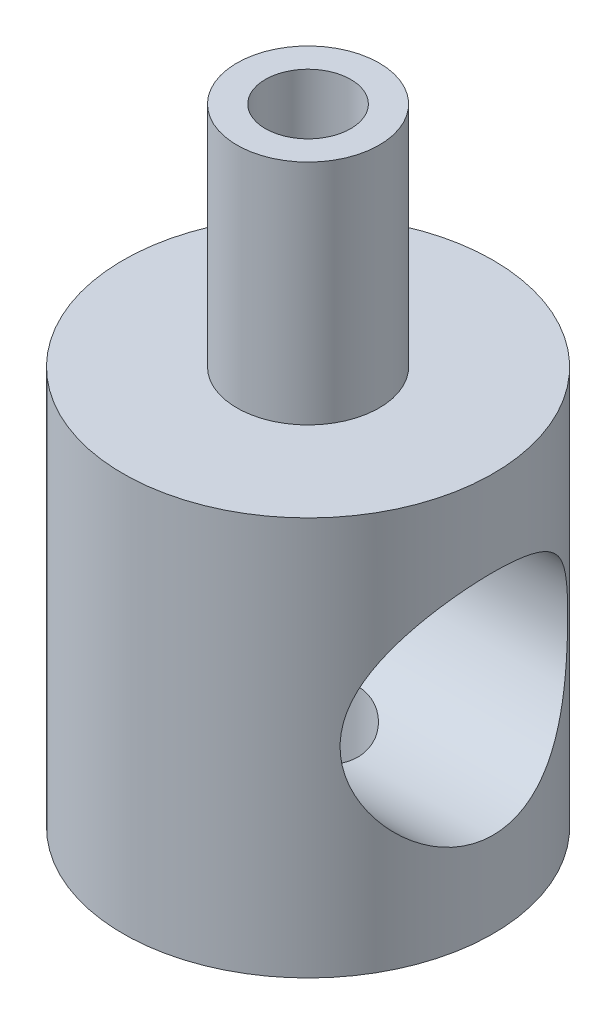
ISO-10303-21;
HEADER;
FILE_DESCRIPTION(('STEP AP214'),'2;1');
FILE_NAME('part.step','',(''),(''),'','','');
FILE_SCHEMA(('AUTOMOTIVE_DESIGN { 1 0 10303 214 1 1 1 1 }'));
ENDSEC;
DATA;
#1=APPLICATION_CONTEXT('core data for automotive mechanical design processes');
#2=APPLICATION_PROTOCOL_DEFINITION('international standard','automotive_design',2000,#1);
#3=PRODUCT_CONTEXT('',#1,'mechanical');
#4=PRODUCT('Part','Part','',(#3));
#5=PRODUCT_RELATED_PRODUCT_CATEGORY('part','',(#4));
#6=PRODUCT_DEFINITION_FORMATION('','',#4);
#7=PRODUCT_DEFINITION_CONTEXT('part definition',#1,'design');
#8=PRODUCT_DEFINITION('design','',#6,#7);
#9=PRODUCT_DEFINITION_SHAPE('','',#8);
#10=(LENGTH_UNIT() NAMED_UNIT(*) SI_UNIT(.MILLI.,.METRE.));
#11=(NAMED_UNIT(*) PLANE_ANGLE_UNIT() SI_UNIT($,.RADIAN.));
#12=(NAMED_UNIT(*) SI_UNIT($,.STERADIAN.) SOLID_ANGLE_UNIT());
#13=UNCERTAINTY_MEASURE_WITH_UNIT(LENGTH_MEASURE(1.E-05),#10,'distance_accuracy_value','');
#14=(GEOMETRIC_REPRESENTATION_CONTEXT(3) GLOBAL_UNCERTAINTY_ASSIGNED_CONTEXT((#13)) GLOBAL_UNIT_ASSIGNED_CONTEXT((#10,
#11,#12)) REPRESENTATION_CONTEXT('',''));
#15=CARTESIAN_POINT('',(0.,0.,0.));
#16=DIRECTION('',(0.,0.,1.));
#17=DIRECTION('',(1.,0.,0.));
#18=AXIS2_PLACEMENT_3D('',#15,#16,#17);
#19=CARTESIAN_POINT('',(6.5,0.,0.));
#20=DIRECTION('',(0.,-1.,0.));
#21=DIRECTION('',(0.,0.,-1.));
#22=AXIS2_PLACEMENT_3D('',#19,#20,#21);
#23=PLANE('',#22);
#24=CARTESIAN_POINT('',(0.,0.,0.));
#25=DIRECTION('',(0.,-1.,0.));
#26=DIRECTION('',(0.,0.,-1.));
#27=AXIS2_PLACEMENT_3D('',#24,#25,#26);
#28=CIRCLE('',#27,1.75);
#29=CARTESIAN_POINT('',(0.,0.,-1.75));
#30=VERTEX_POINT('',#29);
#31=EDGE_CURVE('E87',#30,#30,#28,.T.);
#32=ORIENTED_EDGE('',*,*,#31,.F.);
#33=EDGE_LOOP('',(#32));
#34=FACE_BOUND('',#33,.T.);
#35=CARTESIAN_POINT('',(0.,0.,0.));
#36=DIRECTION('',(0.,-1.,0.));
#37=DIRECTION('',(0.,0.,-1.));
#38=AXIS2_PLACEMENT_3D('',#35,#36,#37);
#39=CIRCLE('',#38,6.5);
#40=CARTESIAN_POINT('',(0.,0.,-6.5));
#41=VERTEX_POINT('',#40);
#42=EDGE_CURVE('E98',#41,#41,#39,.T.);
#43=ORIENTED_EDGE('',*,*,#42,.T.);
#44=EDGE_LOOP('',(#43));
#45=FACE_BOUND('',#44,.T.);
#46=ADVANCED_FACE('F40',(#34,#45),#23,.T.);
#47=CARTESIAN_POINT('',(0.,22.,0.));
#48=DIRECTION('',(0.,1.,0.));
#49=DIRECTION('',(0.,0.,1.));
#50=AXIS2_PLACEMENT_3D('',#47,#48,#49);
#51=PLANE('',#50);
#52=CARTESIAN_POINT('',(0.,22.,0.));
#53=DIRECTION('',(0.,1.,0.));
#54=DIRECTION('',(0.,0.,1.));
#55=AXIS2_PLACEMENT_3D('',#52,#53,#54);
#56=CIRCLE('',#55,1.5);
#57=CARTESIAN_POINT('',(0.,22.,1.5));
#58=VERTEX_POINT('',#57);
#59=EDGE_CURVE('E92',#58,#58,#56,.T.);
#60=ORIENTED_EDGE('',*,*,#59,.F.);
#61=EDGE_LOOP('',(#60));
#62=FACE_BOUND('',#61,.T.);
#63=CARTESIAN_POINT('',(0.,22.,0.));
#64=DIRECTION('',(0.,-1.,0.));
#65=DIRECTION('',(0.,0.,-1.));
#66=AXIS2_PLACEMENT_3D('',#63,#64,#65);
#67=CIRCLE('',#66,2.5);
#68=CARTESIAN_POINT('',(0.,22.,-2.5));
#69=VERTEX_POINT('',#68);
#70=EDGE_CURVE('E10',#69,#69,#67,.T.);
#71=ORIENTED_EDGE('',*,*,#70,.F.);
#72=EDGE_LOOP('',(#71));
#73=FACE_BOUND('',#72,.T.);
#74=ADVANCED_FACE('F111',(#62,#73),#51,.T.);
#75=CARTESIAN_POINT('',(0.,0.,0.));
#76=DIRECTION('',(0.,-1.,0.));
#77=DIRECTION('',(0.,0.,-1.));
#78=AXIS2_PLACEMENT_3D('',#75,#76,#77);
#79=CYLINDRICAL_SURFACE('',#78,2.5);
#80=ORIENTED_EDGE('',*,*,#70,.T.);
#81=EDGE_LOOP('',(#80));
#82=FACE_BOUND('',#81,.T.);
#83=CARTESIAN_POINT('',(0.,14.,0.));
#84=DIRECTION('',(0.,-1.,0.));
#85=DIRECTION('',(0.,0.,-1.));
#86=AXIS2_PLACEMENT_3D('',#83,#84,#85);
#87=CIRCLE('',#86,2.5);
#88=CARTESIAN_POINT('',(0.,14.,-2.5));
#89=VERTEX_POINT('',#88);
#90=EDGE_CURVE('E47',#89,#89,#87,.T.);
#91=ORIENTED_EDGE('',*,*,#90,.F.);
#92=EDGE_LOOP('',(#91));
#93=FACE_BOUND('',#92,.T.);
#94=ADVANCED_FACE('F110',(#82,#93),#79,.T.);
#95=CARTESIAN_POINT('',(2.5,14.,0.));
#96=DIRECTION('',(0.,1.,0.));
#97=DIRECTION('',(0.,0.,1.));
#98=AXIS2_PLACEMENT_3D('',#95,#96,#97);
#99=PLANE('',#98);
#100=ORIENTED_EDGE('',*,*,#90,.T.);
#101=EDGE_LOOP('',(#100));
#102=FACE_BOUND('',#101,.T.);
#103=CARTESIAN_POINT('',(0.,14.,0.));
#104=DIRECTION('',(0.,-1.,0.));
#105=DIRECTION('',(0.,0.,-1.));
#106=AXIS2_PLACEMENT_3D('',#103,#104,#105);
#107=CIRCLE('',#106,6.5);
#108=CARTESIAN_POINT('',(0.,14.,-6.5));
#109=VERTEX_POINT('',#108);
#110=EDGE_CURVE('E53',#109,#109,#107,.T.);
#111=ORIENTED_EDGE('',*,*,#110,.F.);
#112=EDGE_LOOP('',(#111));
#113=FACE_BOUND('',#112,.T.);
#114=ADVANCED_FACE('F104',(#102,#113),#99,.T.);
#115=CARTESIAN_POINT('',(0.,0.,0.));
#116=DIRECTION('',(0.,-1.,0.));
#117=DIRECTION('',(0.,0.,-1.));
#118=AXIS2_PLACEMENT_3D('',#115,#116,#117);
#119=CYLINDRICAL_SURFACE('',#118,6.5);
#120=CARTESIAN_POINT('',(-5.1234753829798,7.,-4.));
#121=CARTESIAN_POINT('',(-5.12347713657616,6.90015669713617,-3.99999887511368));
#122=CARTESIAN_POINT('',(-5.12640682483417,6.80028579053627,-3.99625399732967));
#123=CARTESIAN_POINT('',(-5.13799719570292,6.60139163701732,-3.98134025862972));
#124=CARTESIAN_POINT('',(-5.1466615873077,6.50236898072765,-3.9701665930275));
#125=CARTESIAN_POINT('',(-5.16936573069827,6.30581741824697,-3.9405590608807));
#126=CARTESIAN_POINT('',(-5.18341719303693,6.20829225109523,-3.9221093750139));
#127=CARTESIAN_POINT('',(-5.21631619694594,6.01562931713894,-3.87824609249434));
#128=CARTESIAN_POINT('',(-5.2351661198617,5.92049276156711,-3.85282903764331));
#129=CARTESIAN_POINT('',(-5.2975118930577,5.64121496157163,-3.76713981429484));
#130=CARTESIAN_POINT('',(-5.34704541637303,5.46131227453469,-3.69713461531885));
#131=CARTESIAN_POINT('',(-5.45637608486704,5.11612784646797,-3.53377707470374));
#132=CARTESIAN_POINT('',(-5.51617292067096,4.9508456649488,-3.44042543677516));
#133=CARTESIAN_POINT('',(-5.6486519372425,4.61590906564967,-3.21892377258575));
#134=CARTESIAN_POINT('',(-5.72199980218117,4.44846262921535,-3.08783223309545));
#135=CARTESIAN_POINT('',(-5.86799191617871,4.1360126501527,-2.80046904719545));
#136=CARTESIAN_POINT('',(-5.94063551475959,3.99102828879258,-2.64417611016677));
#137=CARTESIAN_POINT('',(-6.0483243275859,3.78501097210863,-2.38286990663015));
#138=CARTESIAN_POINT('',(-6.08580938951633,3.71517412457287,-2.28568158855732));
#139=CARTESIAN_POINT('',(-6.15757848162021,3.58403886514078,-2.08461055875057));
#140=CARTESIAN_POINT('',(-6.19186384772521,3.52273688447564,-1.98073067176673));
#141=CARTESIAN_POINT('',(-6.2562444343275,3.40934971683696,-1.76688192807704));
#142=CARTESIAN_POINT('',(-6.28634164261803,3.3572601542414,-1.65691599482346));
#143=CARTESIAN_POINT('',(-6.34144803942563,3.26296530629451,-1.43159946565469));
#144=CARTESIAN_POINT('',(-6.3664581180667,3.22075829154191,-1.31624981610916));
#145=CARTESIAN_POINT('',(-6.40838703250716,3.1505670119568,-1.09278967074767));
#146=CARTESIAN_POINT('',(-6.42586235547201,3.12158728585046,-0.985095920594982));
#147=CARTESIAN_POINT('',(-6.45552932860006,3.0726294915698,-0.766973793679369));
#148=CARTESIAN_POINT('',(-6.46772182283343,3.05264998535452,-0.656545856757168));
#149=CARTESIAN_POINT('',(-6.48645425113834,3.02203123627441,-0.434014676552622));
#150=CARTESIAN_POINT('',(-6.49299865161972,3.01138461303053,-0.321912828470646));
#151=CARTESIAN_POINT('',(-6.50024913730255,2.99959241139628,-0.09702857098902));
#152=CARTESIAN_POINT('',(-6.50095586344691,2.99844578996059,0.0157537623365401));
#153=CARTESIAN_POINT('',(-6.49680097681437,3.00519983836845,0.226182592153617));
#154=CARTESIAN_POINT('',(-6.49265447843572,3.01193858094583,0.323882323128413));
#155=CARTESIAN_POINT('',(-6.48003989038484,3.03250994958416,0.518258298369307));
#156=CARTESIAN_POINT('',(-6.47157050163652,3.04634470808205,0.614934226051794));
#157=CARTESIAN_POINT('',(-6.43993788468158,3.09825697913932,0.902326020411392));
#158=CARTESIAN_POINT('',(-6.41054580962105,3.1467491941822,1.09060145777752));
#159=CARTESIAN_POINT('',(-6.33753263883013,3.26948498619312,1.45625882265054));
#160=CARTESIAN_POINT('',(-6.29385686120839,3.34382759576959,1.63359572328174));
#161=CARTESIAN_POINT('',(-6.19570063444803,3.51551091997735,1.9734742197741));
#162=CARTESIAN_POINT('',(-6.14121759534825,3.61285714849984,2.13601225543652));
#163=CARTESIAN_POINT('',(-6.01811329340776,3.84119316866455,2.46301792903409));
#164=CARTESIAN_POINT('',(-5.94857761116338,3.97484440634392,2.62527932595506));
#165=CARTESIAN_POINT('',(-5.80633337570436,4.26512674610548,2.92648326267955));
#166=CARTESIAN_POINT('',(-5.73362042679609,4.42179044126985,3.06539211925788));
#167=CARTESIAN_POINT('',(-5.58247201496418,4.77671769402503,3.33354274624901));
#168=CARTESIAN_POINT('',(-5.50445614718879,4.9777331220786,3.45941006662978));
#169=CARTESIAN_POINT('',(-5.36292828124607,5.40286838184918,3.67501039724317));
#170=CARTESIAN_POINT('',(-5.29938954688106,5.62694449543688,3.76481025437048));
#171=CARTESIAN_POINT('',(-5.2111969568149,6.03299890825635,3.88555185537444));
#172=CARTESIAN_POINT('',(-5.18074475085953,6.21097742366292,3.92569222311964));
#173=CARTESIAN_POINT('',(-5.13813041921935,6.5728050191953,3.98131827949251));
#174=CARTESIAN_POINT('',(-5.12594478044201,6.75664624069647,3.99683566482825));
#175=CARTESIAN_POINT('',(-5.12168600082458,7.12529980106099,4.00229325003938));
#176=CARTESIAN_POINT('',(-5.12965141888962,7.31011332541085,3.99218441424513));
#177=CARTESIAN_POINT('',(-5.16453073692964,7.6748670885276,3.9469473814774));
#178=CARTESIAN_POINT('',(-5.19146010573793,7.85480322430662,3.9117987593589));
#179=CARTESIAN_POINT('',(-5.26018225750345,8.20355272072869,3.81886572423089));
#180=CARTESIAN_POINT('',(-5.30181972845392,8.37246124927834,3.76131722200471));
#181=CARTESIAN_POINT('',(-5.39546702978721,8.69868577182605,3.62570220427766));
#182=CARTESIAN_POINT('',(-5.44748061653257,8.85599753923496,3.54762825488917));
#183=CARTESIAN_POINT('',(-5.56773730356901,9.18575033153292,3.35638015591539));
#184=CARTESIAN_POINT('',(-5.6371970970822,9.35552815453736,3.23937361019164));
#185=CARTESIAN_POINT('',(-5.7779144213707,9.67485662192666,2.98117533428057));
#186=CARTESIAN_POINT('',(-5.84917370734001,9.82438653536047,2.83995914704197));
#187=CARTESIAN_POINT('',(-5.99792993480129,10.1215519065965,2.51230294955814));
#188=CARTESIAN_POINT('',(-6.07478576966285,10.265621071129,2.32226223380833));
#189=CARTESIAN_POINT('',(-6.17981341127997,10.455842708803,2.01780081268138));
#190=CARTESIAN_POINT('',(-6.21312570303109,10.5149565958551,1.91302977376878));
#191=CARTESIAN_POINT('',(-6.27541066154967,10.6239187018636,1.69757398668656));
#192=CARTESIAN_POINT('',(-6.30438605831685,10.6737727545275,1.58689301876128));
#193=CARTESIAN_POINT('',(-6.35540596966367,10.7606297203576,1.36771717286115));
#194=CARTESIAN_POINT('',(-6.37777789582193,10.7982559662326,1.25954523414219));
#195=CARTESIAN_POINT('',(-6.41730693921316,10.864262936453,1.03954242767521));
#196=CARTESIAN_POINT('',(-6.43446703905276,10.8926489494385,0.927713693370167));
#197=CARTESIAN_POINT('',(-6.46305144652246,10.939718705732,0.701401686913855));
#198=CARTESIAN_POINT('',(-6.47448031829465,10.958410169835,0.586920603258315));
#199=CARTESIAN_POINT('',(-6.49125430740733,10.9857873594104,0.356332076611586));
#200=CARTESIAN_POINT('',(-6.49660034488408,10.9944745982013,0.240224882288972));
#201=CARTESIAN_POINT('',(-6.50072100810798,11.0011719315121,0.0241800032833952));
#202=CARTESIAN_POINT('',(-6.50032377647171,11.0005275597033,-0.075703214515176));
#203=CARTESIAN_POINT('',(-6.49494349113715,10.991779451216,-0.275051177742688));
#204=CARTESIAN_POINT('',(-6.48995903188888,10.9836734282492,-0.374515785523159));
#205=CARTESIAN_POINT('',(-6.47552310051639,10.9601119995884,-0.572201216464003));
#206=CARTESIAN_POINT('',(-6.46607350299796,10.9446596780852,-0.670422543840655));
#207=CARTESIAN_POINT('',(-6.44293674493903,10.9066170064448,-0.864977871596928));
#208=CARTESIAN_POINT('',(-6.42924794861747,10.8840239008214,-0.961311128142404));
#209=CARTESIAN_POINT('',(-6.38312478202401,10.8073556163928,-1.24124770417761));
#210=CARTESIAN_POINT('',(-6.34519014963781,10.7436901377319,-1.42142818690046));
#211=CARTESIAN_POINT('',(-6.25739870433962,10.5928789388212,-1.76836086933044));
#212=CARTESIAN_POINT('',(-6.20753967818403,10.5057288592986,-1.93511056850881));
#213=CARTESIAN_POINT('',(-6.09366985599603,10.3001387976256,-2.26971440354609));
#214=CARTESIAN_POINT('',(-6.02871907904727,10.1793609128653,-2.43581096412528));
#215=CARTESIAN_POINT('',(-5.89363170045023,9.91509953245222,-2.74661627133291));
#216=CARTESIAN_POINT('',(-5.82348918099979,9.77158990693547,-2.89130002938076));
#217=CARTESIAN_POINT('',(-5.67394446001722,9.44294281625941,-3.17577814197269));
#218=CARTESIAN_POINT('',(-5.59459938435396,9.25479387397566,-3.31214609552205));
#219=CARTESIAN_POINT('',(-5.44573530175625,8.85482777542316,-3.55159996486829));
#220=CARTESIAN_POINT('',(-5.37620966590185,8.64302676086279,-3.65470839450382));
#221=CARTESIAN_POINT('',(-5.27084090224943,8.2486922907222,-3.80456746957854));
#222=CARTESIAN_POINT('',(-5.23094618875543,8.07011304567992,-3.85875009839216));
#223=CARTESIAN_POINT('',(-5.18416897638833,7.79607694343881,-3.92110216574551));
#224=CARTESIAN_POINT('',(-5.17076120978012,7.70380262502461,-3.9387240346589));
#225=CARTESIAN_POINT('',(-5.1487383288086,7.51770085441489,-3.96747159089492));
#226=CARTESIAN_POINT('',(-5.14012053111059,7.4238743021785,-3.97860091550645));
#227=CARTESIAN_POINT('',(-5.13055281063194,7.27489069320055,-3.99092178272306));
#228=CARTESIAN_POINT('',(-5.12790291115791,7.22001116126916,-3.99432349889887));
#229=CARTESIAN_POINT('',(-5.12436353114302,7.11009057081354,-3.99886315266007));
#230=CARTESIAN_POINT('',(-5.12347441611906,7.05504948112632,-4.00000062021594));
#231=CARTESIAN_POINT('',(-5.1234753829798,7.,-4.));
#232=B_SPLINE_CURVE_WITH_KNOTS('',3,(#120,#121,#122,#123,#124,#125,#126,#127,#128,#129,#130,
#131,#132,#133,#134,#135,#136,#137,#138,#139,#140,#141,#142,#143,#144,#145,#146,#147,#148,#149,
#150,#151,#152,#153,#154,#155,#156,#157,#158,#159,#160,#161,#162,#163,#164,#165,#166,#167,#168,
#169,#170,#171,#172,#173,#174,#175,#176,#177,#178,#179,#180,#181,#182,#183,#184,#185,#186,#187,
#188,#189,#190,#191,#192,#193,#194,#195,#196,#197,#198,#199,#200,#201,#202,#203,#204,#205,#206,
#207,#208,#209,#210,#211,#212,#213,#214,#215,#216,#217,#218,#219,#220,#221,#222,#223,#224,#225,
#226,#227,#228,#229,#230,#231),.UNSPECIFIED.,.T.,.F.,(4,2,2,2,2,2,2,2,2,2,2,2,2,2,2,2,2,2,2,2,2,
2,2,2,2,2,2,2,2,2,2,2,2,2,2,2,2,2,2,2,2,2,2,2,2,2,2,2,2,2,2,2,2,2,2,4),(0.,0.299465847023186,
0.599125566991792,0.89944042278291,1.19990460821029,1.79511322524675,2.39030390361143,
3.06260834820436,3.73548377320047,4.11128507027528,4.48692875482605,4.86239353791694,
5.23779256717747,5.5759578835789,5.91406914927767,6.25191279710496,6.58971935115932,
6.88341191371048,7.17719278611444,7.76417492115995,8.35343101568564,8.94282849646918,
9.60448206829833,10.2670819563898,11.0124413384164,11.7564128362636,12.3089912060134,
12.8608576731458,13.413780931277,13.9671557303272,14.5148536725638,15.0627502534703,
15.7129948273108,16.3639002039922,17.1112891013322,17.4853137026704,17.8591018628049,
18.2086733445076,18.5580443960154,18.9071367774896,19.2561763455443,19.5554587988362,
19.8548329843429,20.1540815946503,20.4534458203018,21.0352824358616,21.6172271279354,
22.2608757283334,22.9052696372282,23.6385367813605,24.3713065199459,24.9412520597774,
25.2256353387176,25.5098591455138,25.6749380032628,25.840051125734),.UNSPECIFIED.);
#233=CARTESIAN_POINT('',(-5.1234753829798,7.,-4.));
#234=VERTEX_POINT('',#233);
#235=EDGE_CURVE('E61',#234,#234,#232,.T.);
#236=ORIENTED_EDGE('',*,*,#235,.F.);
#237=EDGE_LOOP('',(#236));
#238=FACE_BOUND('',#237,.T.);
#239=CARTESIAN_POINT('',(5.1234753829798,7.,-4.));
#240=CARTESIAN_POINT('',(5.12347713657616,7.09984330286383,-3.99999887511368));
#241=CARTESIAN_POINT('',(5.12640682483417,7.19971420946373,-3.99625399732967));
#242=CARTESIAN_POINT('',(5.13799719570292,7.39860836298269,-3.98134025862972));
#243=CARTESIAN_POINT('',(5.1466615873077,7.49763101927235,-3.9701665930275));
#244=CARTESIAN_POINT('',(5.16936573069827,7.69418258175303,-3.9405590608807));
#245=CARTESIAN_POINT('',(5.18341719303693,7.79170774890477,-3.9221093750139));
#246=CARTESIAN_POINT('',(5.21631619694594,7.98437068286106,-3.87824609249434));
#247=CARTESIAN_POINT('',(5.2351661198617,8.07950723843289,-3.85282903764331));
#248=CARTESIAN_POINT('',(5.2975118930577,8.35878503842837,-3.76713981429484));
#249=CARTESIAN_POINT('',(5.34704541637303,8.53868772546531,-3.69713461531885));
#250=CARTESIAN_POINT('',(5.45637608486704,8.88387215353203,-3.53377707470374));
#251=CARTESIAN_POINT('',(5.51617292067096,9.0491543350512,-3.44042543677516));
#252=CARTESIAN_POINT('',(5.6486519372425,9.38409093435033,-3.21892377258575));
#253=CARTESIAN_POINT('',(5.72199980218117,9.55153737078466,-3.08783223309545));
#254=CARTESIAN_POINT('',(5.86799191617871,9.8639873498473,-2.80046904719545));
#255=CARTESIAN_POINT('',(5.94063551475959,10.0089717112074,-2.64417611016677));
#256=CARTESIAN_POINT('',(6.0483243275859,10.2149890278914,-2.38286990663015));
#257=CARTESIAN_POINT('',(6.08580938951633,10.2848258754271,-2.28568158855732));
#258=CARTESIAN_POINT('',(6.15757848162021,10.4159611348592,-2.08461055875056));
#259=CARTESIAN_POINT('',(6.19186384772521,10.4772631155244,-1.98073067176673));
#260=CARTESIAN_POINT('',(6.2562444343275,10.590650283163,-1.76688192807704));
#261=CARTESIAN_POINT('',(6.28634164261803,10.6427398457586,-1.65691599482346));
#262=CARTESIAN_POINT('',(6.34144803942563,10.7370346937055,-1.43159946565469));
#263=CARTESIAN_POINT('',(6.36645811806669,10.7792417084581,-1.31624981610916));
#264=CARTESIAN_POINT('',(6.40838703250716,10.8494329880432,-1.09278967074767));
#265=CARTESIAN_POINT('',(6.42586235547201,10.8784127141495,-0.985095920594983));
#266=CARTESIAN_POINT('',(6.45552932860006,10.9273705084302,-0.766973793679371));
#267=CARTESIAN_POINT('',(6.46772182283343,10.9473500146455,-0.656545856757169));
#268=CARTESIAN_POINT('',(6.48645425113834,10.9779687637256,-0.434014676552623));
#269=CARTESIAN_POINT('',(6.49299865161972,10.9886153869695,-0.321912828470648));
#270=CARTESIAN_POINT('',(6.50024913730255,11.0004075886037,-0.0970285709890214));
#271=CARTESIAN_POINT('',(6.50095586344691,11.0015542100394,0.0157537623365388));
#272=CARTESIAN_POINT('',(6.49680097681437,10.9948001616315,0.226182592153616));
#273=CARTESIAN_POINT('',(6.49265447843572,10.9880614190542,0.323882323128411));
#274=CARTESIAN_POINT('',(6.48003989038484,10.9674900504158,0.518258298369306));
#275=CARTESIAN_POINT('',(6.47157050163652,10.953655291918,0.614934226051793));
#276=CARTESIAN_POINT('',(6.43993788468158,10.9017430208607,0.902326020411391));
#277=CARTESIAN_POINT('',(6.41054580962105,10.8532508058178,1.09060145777752));
#278=CARTESIAN_POINT('',(6.33753263883013,10.7305150138069,1.45625882265053));
#279=CARTESIAN_POINT('',(6.29385686120839,10.6561724042304,1.63359572328174));
#280=CARTESIAN_POINT('',(6.19570063444803,10.4844890800226,1.9734742197741));
#281=CARTESIAN_POINT('',(6.14121759534825,10.3871428515002,2.13601225543652));
#282=CARTESIAN_POINT('',(6.01811329340776,10.1588068313354,2.46301792903408));
#283=CARTESIAN_POINT('',(5.94857761116338,10.0251555936561,2.62527932595506));
#284=CARTESIAN_POINT('',(5.80633337570436,9.73487325389452,2.92648326267955));
#285=CARTESIAN_POINT('',(5.73362042679609,9.57820955873015,3.06539211925788));
#286=CARTESIAN_POINT('',(5.58247201496418,9.22328230597497,3.33354274624901));
#287=CARTESIAN_POINT('',(5.50445614718879,9.02226687792141,3.45941006662977));
#288=CARTESIAN_POINT('',(5.36292828124607,8.59713161815082,3.67501039724316));
#289=CARTESIAN_POINT('',(5.29938954688106,8.37305550456312,3.76481025437048));
#290=CARTESIAN_POINT('',(5.2111969568149,7.96700109174365,3.88555185537444));
#291=CARTESIAN_POINT('',(5.18074475085953,7.78902257633708,3.92569222311964));
#292=CARTESIAN_POINT('',(5.13813041921935,7.4271949808047,3.98131827949251));
#293=CARTESIAN_POINT('',(5.12594478044201,7.24335375930353,3.99683566482825));
#294=CARTESIAN_POINT('',(5.12168600082458,6.87470019893901,4.00229325003938));
#295=CARTESIAN_POINT('',(5.12965141888962,6.68988667458915,3.99218441424513));
#296=CARTESIAN_POINT('',(5.16453073692964,6.3251329114724,3.9469473814774));
#297=CARTESIAN_POINT('',(5.19146010573793,6.14519677569338,3.9117987593589));
#298=CARTESIAN_POINT('',(5.26018225750345,5.79644727927131,3.81886572423089));
#299=CARTESIAN_POINT('',(5.30181972845392,5.62753875072166,3.76131722200471));
#300=CARTESIAN_POINT('',(5.39546702978721,5.30131422817395,3.62570220427766));
#301=CARTESIAN_POINT('',(5.44748061653257,5.14400246076504,3.54762825488917));
#302=CARTESIAN_POINT('',(5.56773730356902,4.81424966846708,3.35638015591539));
#303=CARTESIAN_POINT('',(5.63719709708221,4.64447184546264,3.23937361019164));
#304=CARTESIAN_POINT('',(5.7779144213707,4.32514337807334,2.98117533428057));
#305=CARTESIAN_POINT('',(5.84917370734001,4.17561346463953,2.83995914704196));
#306=CARTESIAN_POINT('',(5.99792993480129,3.87844809340346,2.51230294955814));
#307=CARTESIAN_POINT('',(6.07478576966285,3.734378928871,2.32226223380833));
#308=CARTESIAN_POINT('',(6.17981341127997,3.54415729119696,2.01780081268138));
#309=CARTESIAN_POINT('',(6.21312570303109,3.48504340414485,1.91302977376878));
#310=CARTESIAN_POINT('',(6.27541066154967,3.37608129813636,1.69757398668656));
#311=CARTESIAN_POINT('',(6.30438605831685,3.32622724547246,1.58689301876128));
#312=CARTESIAN_POINT('',(6.35540596966367,3.23937027964238,1.36771717286115));
#313=CARTESIAN_POINT('',(6.37777789582193,3.20174403376744,1.25954523414219));
#314=CARTESIAN_POINT('',(6.41730693921316,3.13573706354701,1.0395424276752));
#315=CARTESIAN_POINT('',(6.43446703905276,3.1073510505615,0.927713693370165));
#316=CARTESIAN_POINT('',(6.46305144652246,3.060281294268,0.701401686913854));
#317=CARTESIAN_POINT('',(6.47448031829465,3.04158983016499,0.586920603258314));
#318=CARTESIAN_POINT('',(6.49125430740733,3.01421264058956,0.356332076611585));
#319=CARTESIAN_POINT('',(6.49660034488408,3.00552540179873,0.240224882288971));
#320=CARTESIAN_POINT('',(6.50072100810798,2.99882806848788,0.0241800032833953));
#321=CARTESIAN_POINT('',(6.50032377647171,2.99947244029669,-0.0757032145151747));
#322=CARTESIAN_POINT('',(6.49494349113715,3.00822054878402,-0.275051177742687));
#323=CARTESIAN_POINT('',(6.48995903188888,3.01632657175076,-0.374515785523159));
#324=CARTESIAN_POINT('',(6.47552310051639,3.03988800041164,-0.572201216464002));
#325=CARTESIAN_POINT('',(6.46607350299796,3.05534032191477,-0.670422543840654));
#326=CARTESIAN_POINT('',(6.44293674493903,3.09338299355516,-0.864977871596926));
#327=CARTESIAN_POINT('',(6.42924794861747,3.1159760991786,-0.961311128142403));
#328=CARTESIAN_POINT('',(6.38312478202401,3.19264438360721,-1.24124770417761));
#329=CARTESIAN_POINT('',(6.34519014963781,3.25630986226808,-1.42142818690046));
#330=CARTESIAN_POINT('',(6.25739870433962,3.40712106117877,-1.76836086933044));
#331=CARTESIAN_POINT('',(6.20753967818403,3.49427114070143,-1.93511056850881));
#332=CARTESIAN_POINT('',(6.09366985599603,3.69986120237435,-2.26971440354609));
#333=CARTESIAN_POINT('',(6.02871907904727,3.8206390871347,-2.43581096412528));
#334=CARTESIAN_POINT('',(5.89363170045023,4.08490046754778,-2.74661627133292));
#335=CARTESIAN_POINT('',(5.82348918099979,4.22841009306453,-2.89130002938076));
#336=CARTESIAN_POINT('',(5.67394446001722,4.5570571837406,-3.17577814197269));
#337=CARTESIAN_POINT('',(5.59459938435396,4.74520612602434,-3.31214609552205));
#338=CARTESIAN_POINT('',(5.44573530175625,5.14517222457684,-3.55159996486829));
#339=CARTESIAN_POINT('',(5.37620966590185,5.35697323913721,-3.65470839450382));
#340=CARTESIAN_POINT('',(5.27084090224943,5.7513077092778,-3.80456746957854));
#341=CARTESIAN_POINT('',(5.23094618875543,5.92988695432008,-3.85875009839216));
#342=CARTESIAN_POINT('',(5.18416897638833,6.20392305656119,-3.92110216574551));
#343=CARTESIAN_POINT('',(5.17076120978012,6.29619737497539,-3.9387240346589));
#344=CARTESIAN_POINT('',(5.1487383288086,6.48229914558511,-3.96747159089492));
#345=CARTESIAN_POINT('',(5.14012053111059,6.5761256978215,-3.97860091550645));
#346=CARTESIAN_POINT('',(5.13055281063194,6.72510930679945,-3.99092178272306));
#347=CARTESIAN_POINT('',(5.12790291115791,6.77998883873085,-3.99432349889887));
#348=CARTESIAN_POINT('',(5.12436353114302,6.88990942918646,-3.99886315266007));
#349=CARTESIAN_POINT('',(5.12347441611906,6.94495051887368,-4.00000062021594));
#350=CARTESIAN_POINT('',(5.1234753829798,7.,-4.));
#351=B_SPLINE_CURVE_WITH_KNOTS('',3,(#239,#240,#241,#242,#243,#244,#245,#246,#247,#248,#249,
#250,#251,#252,#253,#254,#255,#256,#257,#258,#259,#260,#261,#262,#263,#264,#265,#266,#267,#268,
#269,#270,#271,#272,#273,#274,#275,#276,#277,#278,#279,#280,#281,#282,#283,#284,#285,#286,#287,
#288,#289,#290,#291,#292,#293,#294,#295,#296,#297,#298,#299,#300,#301,#302,#303,#304,#305,#306,
#307,#308,#309,#310,#311,#312,#313,#314,#315,#316,#317,#318,#319,#320,#321,#322,#323,#324,#325,
#326,#327,#328,#329,#330,#331,#332,#333,#334,#335,#336,#337,#338,#339,#340,#341,#342,#343,#344,
#345,#346,#347,#348,#349,#350),.UNSPECIFIED.,.T.,.F.,(4,2,2,2,2,2,2,2,2,2,2,2,2,2,2,2,2,2,2,2,2,
2,2,2,2,2,2,2,2,2,2,2,2,2,2,2,2,2,2,2,2,2,2,2,2,2,2,2,2,2,2,2,2,2,2,4),(0.,0.299465847023186,
0.599125566991791,0.899440422782911,1.19990460821029,1.79511322524675,2.39030390361143,
3.06260834820436,3.73548377320047,4.11128507027528,4.48692875482605,4.86239353791694,
5.23779256717747,5.5759578835789,5.91406914927767,6.25191279710495,6.58971935115932,
6.88341191371048,7.17719278611443,7.76417492115995,8.35343101568564,8.94282849646918,
9.60448206829833,10.2670819563898,11.0124413384164,11.7564128362636,12.3089912060134,
12.8608576731458,13.413780931277,13.9671557303272,14.5148536725638,15.0627502534703,
15.7129948273108,16.3639002039922,17.1112891013322,17.4853137026704,17.8591018628049,
18.2086733445076,18.5580443960154,18.9071367774896,19.2561763455443,19.5554587988362,
19.8548329843429,20.1540815946503,20.4534458203018,21.0352824358616,21.6172271279354,
22.2608757283334,22.9052696372282,23.6385367813605,24.3713065199459,24.9412520597774,
25.2256353387176,25.5098591455138,25.6749380032628,25.840051125734),.UNSPECIFIED.);
#352=CARTESIAN_POINT('',(5.1234753829798,7.,-4.));
#353=VERTEX_POINT('',#352);
#354=EDGE_CURVE('E59',#353,#353,#351,.T.);
#355=ORIENTED_EDGE('',*,*,#354,.F.);
#356=EDGE_LOOP('',(#355));
#357=FACE_BOUND('',#356,.T.);
#358=ORIENTED_EDGE('',*,*,#110,.T.);
#359=EDGE_LOOP('',(#358));
#360=FACE_BOUND('',#359,.T.);
#361=ORIENTED_EDGE('',*,*,#42,.F.);
#362=EDGE_LOOP('',(#361));
#363=FACE_BOUND('',#362,.T.);
#364=ADVANCED_FACE('F68',(#238,#357,#360,#363),#119,.T.);
#365=CARTESIAN_POINT('',(-44.,7.,0.));
#366=DIRECTION('',(1.,0.,0.));
#367=DIRECTION('',(0.,0.,-1.));
#368=AXIS2_PLACEMENT_3D('',#365,#366,#367);
#369=CYLINDRICAL_SURFACE('',#368,4.);
#370=CARTESIAN_POINT('',(0.,10.7080992435478,1.5));
#371=CARTESIAN_POINT('',(0.0810074837207898,10.7080964063381,1.50000304106109));
#372=CARTESIAN_POINT('',(0.161994922503636,10.7107826024099,1.49341597549487));
#373=CARTESIAN_POINT('',(0.321528082913202,10.7211615930497,1.46736187895468));
#374=CARTESIAN_POINT('',(0.400073877595012,10.7288542376711,1.44789523373263));
#375=CARTESIAN_POINT('',(0.552375371613527,10.748254802809,1.39689657610574));
#376=CARTESIAN_POINT('',(0.626142056651084,10.7599530956926,1.36539347266348));
#377=CARTESIAN_POINT('',(0.76737189681884,10.786031342066,1.29131856742698));
#378=CARTESIAN_POINT('',(0.83483315028252,10.8004121006732,1.24874344095039));
#379=CARTESIAN_POINT('',(0.964890311622818,10.8310357466571,1.15146661374162));
#380=CARTESIAN_POINT('',(1.02712852962939,10.847333419236,1.09630381213306));
#381=CARTESIAN_POINT('',(1.14172281467149,10.8794975062855,0.976395839778926));
#382=CARTESIAN_POINT('',(1.19407677374185,10.8953638281478,0.911648630256679));
#383=CARTESIAN_POINT('',(1.28913951229561,10.9255287393655,0.7716946551776));
#384=CARTESIAN_POINT('',(1.33145947471586,10.9397556122351,0.696206947538027));
#385=CARTESIAN_POINT('',(1.40265117252491,10.9643800797385,0.538555771965246));
#386=CARTESIAN_POINT('',(1.43152757199198,10.9747790021701,0.456394630933535));
#387=CARTESIAN_POINT('',(1.47375789577462,10.9901869710344,0.291489341676831));
#388=CARTESIAN_POINT('',(1.48772762744046,10.9954091521477,0.208923197281595));
#389=CARTESIAN_POINT('',(1.50172120094499,11.0006401410794,0.042464363794785));
#390=CARTESIAN_POINT('',(1.50174957761871,11.000650644149,-0.041427885062834));
#391=CARTESIAN_POINT('',(1.48821823853483,10.9955926590389,-0.203743543064477));
#392=CARTESIAN_POINT('',(1.47533070205119,10.9907754199668,-0.282232178266901));
#393=CARTESIAN_POINT('',(1.43746408477445,10.9769327493226,-0.435839217984392));
#394=CARTESIAN_POINT('',(1.41248414773796,10.9679070197558,-0.510957383430299));
#395=CARTESIAN_POINT('',(1.35082954832415,10.9463776916753,-0.656989017303105));
#396=CARTESIAN_POINT('',(1.31398999473159,10.9338253947008,-0.72782539228731));
#397=CARTESIAN_POINT('',(1.22980790307061,10.9065131022528,-0.86248660795756));
#398=CARTESIAN_POINT('',(1.1824619769824,10.8917523951284,-0.926309176932324));
#399=CARTESIAN_POINT('',(1.07537271371681,10.8605252965582,-1.04909048680094));
#400=CARTESIAN_POINT('',(1.01506608434957,10.8440096376388,-1.10754614526348));
#401=CARTESIAN_POINT('',(0.885407006678439,10.8118246064572,-1.21370395569342));
#402=CARTESIAN_POINT('',(0.816052293413359,10.7961554474885,-1.261403406929));
#403=CARTESIAN_POINT('',(0.668280532537176,10.7671270350034,-1.34565611808152));
#404=CARTESIAN_POINT('',(0.589696506313931,10.7538267715028,-1.38193847851831));
#405=CARTESIAN_POINT('',(0.426903774832425,10.73172438629,-1.44056464441501));
#406=CARTESIAN_POINT('',(0.342698228406307,10.7229197620578,-1.46291620605595));
#407=CARTESIAN_POINT('',(0.176024037684045,10.7113959722285,-1.49190191709668));
#408=CARTESIAN_POINT('',(0.093715894463857,10.7083678524154,-1.49933521158966));
#409=CARTESIAN_POINT('',(-0.0710093567417441,10.7078653952502,-1.50057885636272));
#410=CARTESIAN_POINT('',(-0.153426432352472,10.7103896700399,-1.49439261093762));
#411=CARTESIAN_POINT('',(-0.311929922287682,10.7203938162974,-1.46929733520157));
#412=CARTESIAN_POINT('',(-0.388131135764662,10.7276327621645,-1.45100618334224));
#413=CARTESIAN_POINT('',(-0.536347944720195,10.7459648704636,-1.40299774640637));
#414=CARTESIAN_POINT('',(-0.608362679168136,10.7570588225017,-1.37327812034623));
#415=CARTESIAN_POINT('',(-0.749164438076206,10.7823624311608,-1.30200292275278));
#416=CARTESIAN_POINT('',(-0.81772929213734,10.7966732889206,-1.26004545177047));
#417=CARTESIAN_POINT('',(-0.94712898172604,10.8266281429429,-1.16591317862479));
#418=CARTESIAN_POINT('',(-1.00796097462463,10.8422726259408,-1.11373463696435));
#419=CARTESIAN_POINT('',(-1.1241683731951,10.8743304655318,-0.996727340900937));
#420=CARTESIAN_POINT('',(-1.17895340876875,10.8907296935703,-0.931306341491061));
#421=CARTESIAN_POINT('',(-1.27683836758944,10.921498749633,-0.79179747175315));
#422=CARTESIAN_POINT('',(-1.31993825294584,10.9358685710766,-0.717709573322672));
#423=CARTESIAN_POINT('',(-1.39294605619961,10.9609498570455,-0.563016329468476));
#424=CARTESIAN_POINT('',(-1.4228991237926,10.9716738133801,-0.482434433064626));
#425=CARTESIAN_POINT('',(-1.46865641384992,10.9882943671257,-0.316881887523254));
#426=CARTESIAN_POINT('',(-1.4844672854224,10.9941932329941,-0.231913320723592));
#427=CARTESIAN_POINT('',(-1.50077440275483,11.0002840731707,-0.0653355852738145));
#428=CARTESIAN_POINT('',(-1.50210948305899,11.0007886095376,0.0161807680608464));
#429=CARTESIAN_POINT('',(-1.49158484055461,10.9968488980922,0.178226786412425));
#430=CARTESIAN_POINT('',(-1.47972670911414,10.9924052471313,0.258756569245258));
#431=CARTESIAN_POINT('',(-1.44374114850638,10.9792108960377,0.414548248377127));
#432=CARTESIAN_POINT('',(-1.41992009412164,10.9705679137802,0.489890731068835));
#433=CARTESIAN_POINT('',(-1.36098998661564,10.9498778362099,0.635515473006391));
#434=CARTESIAN_POINT('',(-1.32587879669525,10.9378300965566,0.705796771275543));
#435=CARTESIAN_POINT('',(-1.24368605649519,10.9109061830007,0.842540176994414));
#436=CARTESIAN_POINT('',(-1.19616335948585,10.8959324010883,0.90871754884685));
#437=CARTESIAN_POINT('',(-1.09119216981239,10.8649950769484,1.03241734752336));
#438=CARTESIAN_POINT('',(-1.03374013419212,10.8490311827403,1.0899366712559));
#439=CARTESIAN_POINT('',(-0.906935868354939,10.8168812973918,1.19781214236196));
#440=CARTESIAN_POINT('',(-0.837115597845688,10.8007280534916,1.24762999816025));
#441=CARTESIAN_POINT('',(-0.689584130426674,10.7709832500364,1.33484709556843));
#442=CARTESIAN_POINT('',(-0.611872115946518,10.7573919563122,1.37224504878157));
#443=CARTESIAN_POINT('',(-0.447044319024594,10.7340226985327,1.4346588697426));
#444=CARTESIAN_POINT('',(-0.359665633488216,10.7244380329086,1.45906002899523));
#445=CARTESIAN_POINT('',(-0.181514728044213,10.7114799433632,1.49172356722079));
#446=CARTESIAN_POINT('',(-0.0907447872900078,10.7081024217974,1.49999659339571));
#447=CARTESIAN_POINT('',(0.,10.7080992435478,1.5));
#448=B_SPLINE_CURVE_WITH_KNOTS('',3,(#370,#371,#372,#373,#374,#375,#376,#377,#378,#379,#380,
#381,#382,#383,#384,#385,#386,#387,#388,#389,#390,#391,#392,#393,#394,#395,#396,#397,#398,#399,
#400,#401,#402,#403,#404,#405,#406,#407,#408,#409,#410,#411,#412,#413,#414,#415,#416,#417,#418,
#419,#420,#421,#422,#423,#424,#425,#426,#427,#428,#429,#430,#431,#432,#433,#434,#435,#436,#437,
#438,#439,#440,#441,#442,#443,#444,#445,#446,#447),.UNSPECIFIED.,.T.,.F.,(4,2,2,2,2,2,2,2,2,2,2,
2,2,2,2,2,2,2,2,2,2,2,2,2,2,2,2,2,2,2,2,2,2,2,2,2,2,2,4),(0.,0.24268454141617,0.485361814598854,
0.72745985675703,0.969630679682933,1.22274652401128,1.47591628822983,1.73770072136421,
1.9993942638133,2.24980018489679,2.50012465404857,2.73806472803194,2.97602165263335,
3.21744131210668,3.45893893628976,3.71456675065875,3.97025867827335,4.23162592252966,
4.49284751635474,4.73965657740485,4.98640395388884,5.22143845928199,5.45652113429526,
5.70041561005821,5.94439948466355,6.20385016993624,6.46330169650178,6.72185508890168,
6.98028685560127,7.22365720549936,7.46699820319479,7.7044027400389,7.94185223512831,
8.18928323676987,8.43680270894964,8.69738599542079,8.95799630544242,9.23003178870926,
9.50188762323053),.UNSPECIFIED.);
#449=CARTESIAN_POINT('',(0.,10.7080992435478,1.5));
#450=VERTEX_POINT('',#449);
#451=EDGE_CURVE('E37',#450,#450,#448,.T.);
#452=ORIENTED_EDGE('',*,*,#451,.T.);
#453=EDGE_LOOP('',(#452));
#454=FACE_BOUND('',#453,.T.);
#455=CARTESIAN_POINT('',(0.,3.40312635751546,-1.75));
#456=CARTESIAN_POINT('',(0.0928371055771344,3.40312180545111,-1.74999577608997));
#457=CARTESIAN_POINT('',(0.185828428803379,3.39948012528176,-1.74256561547484));
#458=CARTESIAN_POINT('',(0.369085319059166,3.3854017865309,-1.71316453984274));
#459=CARTESIAN_POINT('',(0.459343214333317,3.37494757820629,-1.69115606723878));
#460=CARTESIAN_POINT('',(0.634153944624203,3.34867035591395,-1.63363928523817));
#461=CARTESIAN_POINT('',(0.718729791646312,3.33287078635513,-1.59818984646979));
#462=CARTESIAN_POINT('',(0.880711383150333,3.29771864761208,-1.5149738058054));
#463=CARTESIAN_POINT('',(0.958118311786913,3.278366666792,-1.46720924305884));
#464=CARTESIAN_POINT('',(1.10893120241348,3.23680375473651,-1.3572089262902));
#465=CARTESIAN_POINT('',(1.18178602073876,3.2144897743871,-1.29425610425353));
#466=CARTESIAN_POINT('',(1.31631644989053,3.17035980368035,-1.15716879759801));
#467=CARTESIAN_POINT('',(1.37798748518343,3.14854402032255,-1.08302975907306));
#468=CARTESIAN_POINT('',(1.49131486343688,3.10659385789064,-0.921247017509311));
#469=CARTESIAN_POINT('',(1.54233744195333,3.08659305224905,-0.833121556719551));
#470=CARTESIAN_POINT('',(1.62859114853938,3.05180481242705,-0.648503189012278));
#471=CARTESIAN_POINT('',(1.66382996951412,3.03701483927111,-0.552014385765683));
#472=CARTESIAN_POINT('',(1.71547580606914,3.01504796698644,-0.359208082434876));
#473=CARTESIAN_POINT('',(1.73283696114782,3.0074870887074,-0.263190827254633));
#474=CARTESIAN_POINT('',(1.75133162189587,2.99942647863167,-0.0693287873971891));
#475=CARTESIAN_POINT('',(1.75247243077953,2.99892356898444,0.0285151549420435));
#476=CARTESIAN_POINT('',(1.73896359566614,3.00481953496087,0.216261746914355));
#477=CARTESIAN_POINT('',(1.72536634083182,3.01075844524396,0.306257390419992));
#478=CARTESIAN_POINT('',(1.6845897501027,3.0282239977533,0.482538817916277));
#479=CARTESIAN_POINT('',(1.65740940914617,3.03975105346477,0.568824326867456));
#480=CARTESIAN_POINT('',(1.58993643773862,3.06751463416614,0.736835262665255));
#481=CARTESIAN_POINT('',(1.54944971226715,3.08382045877576,0.818470815688342));
#482=CARTESIAN_POINT('',(1.45671622723929,3.1195755588594,0.974004107270158));
#483=CARTESIAN_POINT('',(1.40446520371499,3.13902597336704,1.0478990259724));
#484=CARTESIAN_POINT('',(1.28504671238787,3.18090517281334,1.19187174309814));
#485=CARTESIAN_POINT('',(1.21704346368027,3.20344797447906,1.26122407671226));
#486=CARTESIAN_POINT('',(1.0703744239086,3.24789117727666,1.38787377204875));
#487=CARTESIAN_POINT('',(0.991703669426825,3.26979127356369,1.44516549029935));
#488=CARTESIAN_POINT('',(0.82205739941348,3.3113327845053,1.54820801514461));
#489=CARTESIAN_POINT('',(0.730719618204054,3.33085148178365,1.59341626667799));
#490=CARTESIAN_POINT('',(0.540649902454669,3.36391885569972,1.6675068498565));
#491=CARTESIAN_POINT('',(0.441923951900663,3.37747230390101,1.69640223530589));
#492=CARTESIAN_POINT('',(0.247169299223133,3.39585485518718,1.73509908818066));
#493=CARTESIAN_POINT('',(0.151428096754178,3.40122364486126,1.74608539056461));
#494=CARTESIAN_POINT('',(-0.04066000344493,3.40417632746755,1.75216137559478));
#495=CARTESIAN_POINT('',(-0.137006636912355,3.40176340941232,1.74725757014364));
#496=CARTESIAN_POINT('',(-0.32006311438135,3.3899865811515,1.72277634072846));
#497=CARTESIAN_POINT('',(-0.406959642818104,3.38114842012903,1.70430774610854));
#498=CARTESIAN_POINT('',(-0.576329409152534,3.35821404842456,1.65473120013592));
#499=CARTESIAN_POINT('',(-0.658801534061002,3.34411652174126,1.62362008519095));
#500=CARTESIAN_POINT('',(-0.821070870840737,3.3114972183598,1.54812910706366));
#501=CARTESIAN_POINT('',(-0.900588450177906,3.29280734187085,1.50322324911612));
#502=CARTESIAN_POINT('',(-1.05136547846522,3.25332627013148,1.40192319593043));
#503=CARTESIAN_POINT('',(-1.12262109004358,3.23253410677459,1.3455236955994));
#504=CARTESIAN_POINT('',(-1.26164578778334,3.18889779543651,1.21676814254937));
#505=CARTESIAN_POINT('',(-1.32849960194522,3.16603993465769,1.14342436340306));
#506=CARTESIAN_POINT('',(-1.44914428383617,3.12258498980563,0.986057837403049));
#507=CARTESIAN_POINT('',(-1.50293355077419,3.10198818294724,0.902033783821306));
#508=CARTESIAN_POINT('',(-1.59608462508259,3.06513791845804,0.724645877674746));
#509=CARTESIAN_POINT('',(-1.63534455814212,3.04891533853879,0.631221708208402));
#510=CARTESIAN_POINT('',(-1.69727435093143,3.02288506710917,0.43819459444585));
#511=CARTESIAN_POINT('',(-1.71995520928519,3.0130731232171,0.338595794094049));
#512=CARTESIAN_POINT('',(-1.74659696219071,3.00150375772961,0.144182360918349));
#513=CARTESIAN_POINT('',(-1.7518444556949,2.9991930637498,0.0495759598119035));
#514=CARTESIAN_POINT('',(-1.74700897845425,3.00130849231806,-0.139156361955344));
#515=CARTESIAN_POINT('',(-1.73692921003997,3.00573320763475,-0.233282378860698));
#516=CARTESIAN_POINT('',(-1.70264619700566,3.02051748543084,-0.414279177098124));
#517=CARTESIAN_POINT('',(-1.67905438139825,3.03061978437695,-0.501288619826495));
#518=CARTESIAN_POINT('',(-1.61911919383194,3.05559800144143,-0.67005721694163));
#519=CARTESIAN_POINT('',(-1.58277353569061,3.07047477536461,-0.751815426911259));
#520=CARTESIAN_POINT('',(-1.49652265103245,3.10443340373007,-0.911900823969187));
#521=CARTESIAN_POINT('',(-1.44607267885892,3.12367663294461,-0.989899416247833));
#522=CARTESIAN_POINT('',(-1.33380569373778,3.16414314553278,-1.13666500542713));
#523=CARTESIAN_POINT('',(-1.27198399894363,3.18536724266915,-1.20542817976969));
#524=CARTESIAN_POINT('',(-1.1332043029573,3.22945590226236,-1.33723149580577));
#525=CARTESIAN_POINT('',(-1.05545252420228,3.25232241116776,-1.3994380988651));
#526=CARTESIAN_POINT('',(-0.889968096990073,3.29551941745171,-1.5100873956313));
#527=CARTESIAN_POINT('',(-0.802229462613692,3.31584837840902,-1.55852177306422));
#528=CARTESIAN_POINT('',(-0.618760029698182,3.35140239984001,-1.64003866605434));
#529=CARTESIAN_POINT('',(-0.523019408881211,3.3666210691223,-1.67310197748509));
#530=CARTESIAN_POINT('',(-0.326594705515189,3.38963379317287,-1.72221188407887));
#531=CARTESIAN_POINT('',(-0.225928409501895,3.39745274813007,-1.73831556951834));
#532=CARTESIAN_POINT('',(-0.10393550397992,3.40168592543117,-1.74703572559822));
#533=CARTESIAN_POINT('',(-0.0831699129497893,3.40222497653118,-1.74814627318149));
#534=CARTESIAN_POINT('',(-0.041605463857901,3.40294570662991,-1.74962889188203));
#535=CARTESIAN_POINT('',(-0.0208066050703023,3.40312737772182,-1.75000094666058));
#536=CARTESIAN_POINT('',(0.,3.40312635751546,-1.75));
#537=B_SPLINE_CURVE_WITH_KNOTS('',3,(#455,#456,#457,#458,#459,#460,#461,#462,#463,#464,#465,
#466,#467,#468,#469,#470,#471,#472,#473,#474,#475,#476,#477,#478,#479,#480,#481,#482,#483,#484,
#485,#486,#487,#488,#489,#490,#491,#492,#493,#494,#495,#496,#497,#498,#499,#500,#501,#502,#503,
#504,#505,#506,#507,#508,#509,#510,#511,#512,#513,#514,#515,#516,#517,#518,#519,#520,#521,#522,
#523,#524,#525,#526,#527,#528,#529,#530,#531,#532,#533,#534,#535,#536),.UNSPECIFIED.,.T.,.F.,(4,
2,2,2,2,2,2,2,2,2,2,2,2,2,2,2,2,2,2,2,2,2,2,2,2,2,2,2,2,2,2,2,2,2,2,2,2,2,2,2,4),(0.,
0.278423709089657,0.557567515667148,0.83550255411435,1.11339160134649,1.40862253901942,
1.703973991051,2.01370508313311,2.32328504950115,2.6153188205415,2.90722109914898,
3.17957432675714,3.45194770975124,3.72848484888748,4.00512238068054,4.30294103546421,
4.60089873899835,4.91057566441317,5.22000442909256,5.50798165433932,5.79584087897396,
6.06247089944839,6.32916768102552,6.60765996633827,6.88628108699589,7.19039073128141,
7.49453761916006,7.80077838726026,8.10681580917881,8.38969680616703,8.67251870884305,
8.94345335784295,9.21443659790207,9.49782974545364,9.78133983087841,10.0864214236492,
10.3916868487401,10.6973326446402,11.0019462404003,11.0643450405093,11.12674522114),.UNSPECIFIED.);
#538=CARTESIAN_POINT('',(0.,3.40312635751546,-1.75));
#539=VERTEX_POINT('',#538);
#540=EDGE_CURVE('E67',#539,#539,#537,.T.);
#541=ORIENTED_EDGE('',*,*,#540,.T.);
#542=EDGE_LOOP('',(#541));
#543=FACE_BOUND('',#542,.T.);
#544=ORIENTED_EDGE('',*,*,#235,.T.);
#545=EDGE_LOOP('',(#544));
#546=FACE_BOUND('',#545,.T.);
#547=ORIENTED_EDGE('',*,*,#354,.T.);
#548=EDGE_LOOP('',(#547));
#549=FACE_BOUND('',#548,.T.);
#550=ADVANCED_FACE('F71',(#454,#543,#546,#549),#369,.F.);
#551=CARTESIAN_POINT('',(0.,4.99999999999998,0.));
#552=DIRECTION('',(0.,-1.,0.));
#553=DIRECTION('',(0.,0.,-1.));
#554=AXIS2_PLACEMENT_3D('',#551,#552,#553);
#555=CYLINDRICAL_SURFACE('',#554,1.75);
#556=ORIENTED_EDGE('',*,*,#31,.T.);
#557=EDGE_LOOP('',(#556));
#558=FACE_BOUND('',#557,.T.);
#559=ORIENTED_EDGE('',*,*,#540,.F.);
#560=EDGE_LOOP('',(#559));
#561=FACE_BOUND('',#560,.T.);
#562=ADVANCED_FACE('F79',(#558,#561),#555,.F.);
#563=CARTESIAN_POINT('',(0.,9.00000000000002,0.));
#564=DIRECTION('',(0.,1.,0.));
#565=DIRECTION('',(0.,0.,1.));
#566=AXIS2_PLACEMENT_3D('',#563,#564,#565);
#567=CYLINDRICAL_SURFACE('',#566,1.5);
#568=ORIENTED_EDGE('',*,*,#59,.T.);
#569=EDGE_LOOP('',(#568));
#570=FACE_BOUND('',#569,.T.);
#571=ORIENTED_EDGE('',*,*,#451,.F.);
#572=EDGE_LOOP('',(#571));
#573=FACE_BOUND('',#572,.T.);
#574=ADVANCED_FACE('F133',(#570,#573),#567,.F.);
#575=CLOSED_SHELL('',(#46,#74,#94,#114,#364,#550,#562,#574));
#576=MANIFOLD_SOLID_BREP('B2',#575);
#577=ADVANCED_BREP_SHAPE_REPRESENTATION('',(#18,#576),#14);
#578=SHAPE_DEFINITION_REPRESENTATION(#9,#577);
ENDSEC;
END-ISO-10303-21;
